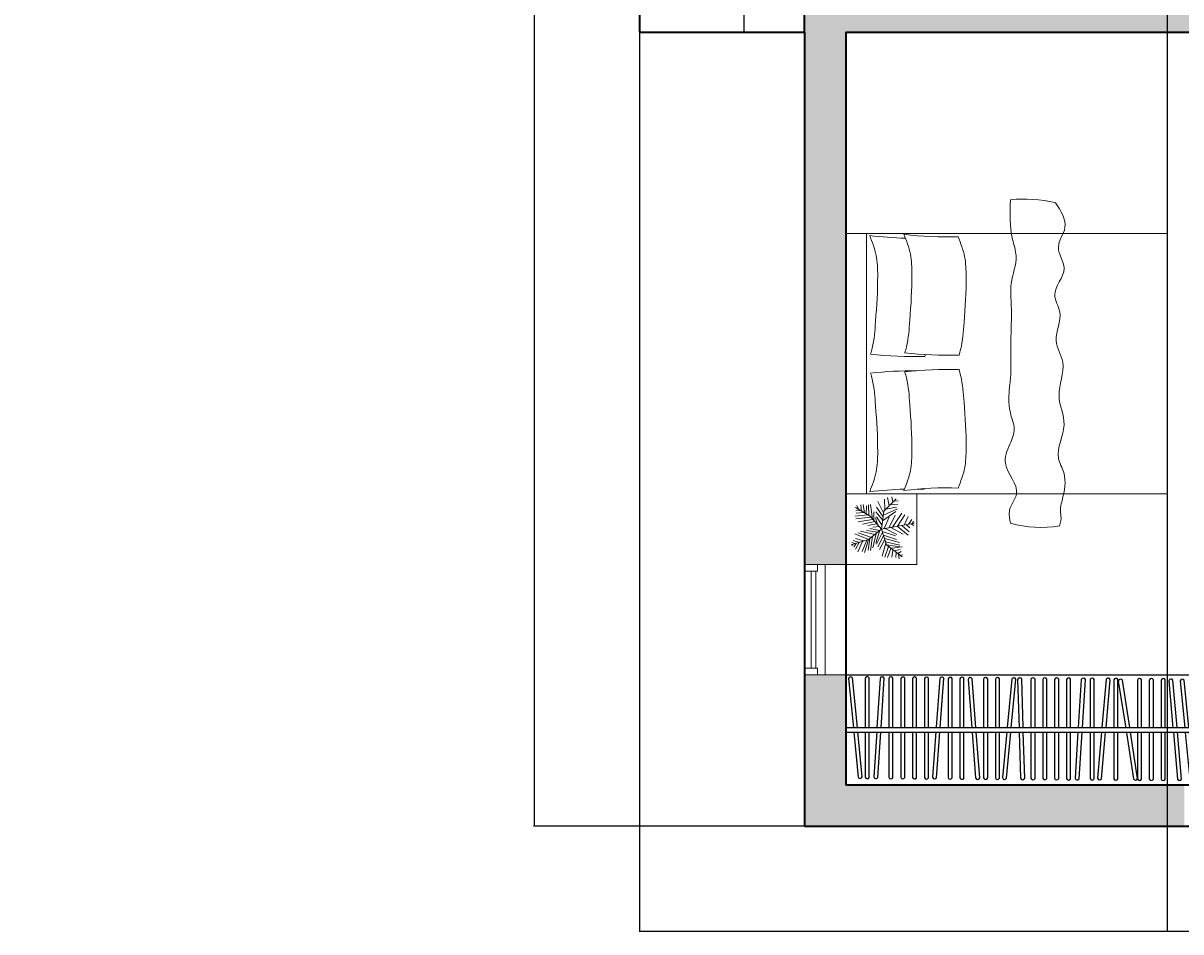
# Model space of a CAD drawing. Units: inches. Extents: x 1789 to 2841, y 3180 to 3702.
# Tile 1 of 14: x 1789 to 2041, y 3180 to 3378. Entities that reach past the tile are written whole.
import ezdxf

# ---------------------------------------------------------------- set-up
doc = ezdxf.new("R2010")
doc.units = ezdxf.units.IN
doc.header["$MEASUREMENT"] = 0
for name, color, linetype, lineweight in [('A-ANNO-DIMS', 2, 'Continuous', 18), ('A-FLOR-CASE', 34, 'Continuous', 25), ('A-WALL', 40, 'Continuous', 35), ('A-WALL-PATT', 252, 'Continuous', 13), ('FURNITURE', 34, 'Continuous', 18), ('WINDOWS', 130, 'Continuous', 18)]:
    doc.layers.add(name, color=color, linetype=linetype, lineweight=lineweight)
doc.styles.get("Standard").update_dxf_attribs({"font": 'arial.ttf'})
doc.dimstyles.get("Standard").update_dxf_attribs({"dimtxt": 0.18, "dimasz": 0.18, "dimexe": 0.18, "dimexo": 0.0625, "dimgap": 0.09, "dimtad": 0, "dimtih": 1, "dimtoh": 1, "dimdec": 0, "dimzin": 0, "dimdsep": 46, "dimlunit": 3, "dimtxsty": 'Standard', "dimcen": 0.09, "dimadec": 0, "dimazin": 0, "dimtfac": 1, "dimtdec": 0, "dimtofl": 0, "dimtmove": 0, "dimatfit": 3, "dimfxl": 1, "dimtolj": 1, "dimtzin": 0, "dimarcsym": 0})

# ---------------------------------------------------------------- blocks, each defined once
blk = doc.blocks.new('CUBOARD')
for p, q in [((2183.73, 3646.16), (2183.73, 3568.16)), ((2184.71, 3646.16), (2184.71, 3568.16))]:
    blk.add_line(p, q)
blk.add_lwpolyline([(2172.23, 3646.16), (2196.23, 3646.16), (2196.23, 3568.16), (2172.23, 3568.16)], close=True)
for points in [[(2183.69, 3644.46), (2173.95, 3643.51)], [(2195.39, 3645.6), (2184.67, 3644.55)], [(2184.76, 3643.66), (2195.54, 3644.71)], [(2195.78, 3645.16), (2195.78, 3645.18)], [(2183.73, 3641.98), (2173.93, 3641.98)], [(2173.97, 3642.61), (2183.78, 3643.57)], [(2195.47, 3641.98), (2184.71, 3641.98)], [(2173.84, 3639.19), (2183.7, 3638.57)], [(2173.86, 3641.08), (2183.73, 3641.08)], [(2183.76, 3639.46), (2173.96, 3640.08)], [(2184.71, 3641.08), (2195.53, 3641.08)], [(2195.45, 3638.71), (2184.74, 3639.4)], [(2195.82, 3641.5), (2195.82, 3641.53)], [(2183.73, 3636.82), (2173.9, 3636.82)], [(2184.68, 3638.5), (2195.46, 3637.81)], [(2195.43, 3636.82), (2184.71, 3636.82)], [(2195.77, 3638.22), (2195.78, 3638.24)], [(2173.83, 3635.92), (2183.73, 3635.92)], [(2183.73, 3634.24), (2173.88, 3634.24)], [(2184.71, 3635.92), (2195.5, 3635.92)], [(2195.42, 3634.24), (2184.71, 3634.24)], [(2195.78, 3636.35), (2195.78, 3636.37)], [(2173.81, 3633.34), (2183.73, 3633.34)], [(2183.73, 3631.66), (2173.86, 3631.66)], [(2184.71, 3633.34), (2195.48, 3633.34)], [(2195.4, 3631.66), (2184.71, 3631.66)], [(2195.77, 3633.77), (2195.77, 3633.79)], [(2173.8, 3630.76), (2183.73, 3630.76)], [(2183.73, 3629.08), (2173.85, 3629.08)], [(2184.71, 3630.76), (2195.47, 3630.76)], [(2195.38, 3629.08), (2184.71, 3629.08)], [(2195.75, 3631.19), (2195.75, 3631.21)], [(2173.78, 3628.19), (2183.73, 3628.19)], [(2183.8, 3626.57), (2173.93, 3627.31)], [(2184.71, 3628.19), (2195.45, 3628.19)], [(2195.4, 3625.7), (2184.78, 3626.5)], [(2195.73, 3628.61), (2195.73, 3628.63)], [(2173.79, 3626.43), (2183.74, 3625.68)], [(2184.71, 3625.61), (2195.4, 3624.81)], [(2195.72, 3625.21), (2195.72, 3625.23)], [(2173.75, 3623.03), (2183.73, 3623.03)], [(2183.73, 3623.92), (2173.81, 3623.92)], [(2195.35, 3623.92), (2184.71, 3623.92)], [(2184.71, 3623.03), (2195.42, 3623.03)], [(2195.7, 3623.45), (2195.7, 3623.48)], [(2173.73, 3620.45), (2183.73, 3620.45)], [(2183.73, 3621.34), (2173.8, 3621.34)], [(2195.22, 3619.57), (2184.65, 3618.76)], [(2195.33, 3621.34), (2184.71, 3621.34)], [(2184.71, 3620.45), (2195.4, 3620.45)], [(2195.6, 3619.13), (2195.6, 3619.15)], [(2195.68, 3620.87), (2195.68, 3620.9)], [(2183.67, 3618.69), (2173.75, 3617.93)], [(2173.75, 3617.03), (2183.74, 3617.8)], [(2184.71, 3617.87), (2195.35, 3618.68)], [(2173.7, 3615.29), (2183.73, 3615.29)], [(2183.73, 3616.19), (2173.77, 3616.19)], [(2195.3, 3616.19), (2184.71, 3616.19)], [(2184.71, 3615.29), (2195.37, 3615.29)], [(2195.65, 3615.71), (2195.65, 3615.74)], [(2173.68, 3612.71), (2183.73, 3612.71)], [(2183.73, 3613.61), (2173.75, 3613.61)], [(2183.78, 3611.12), (2173.82, 3612.07)], [(2195.28, 3613.61), (2184.71, 3613.61)], [(2184.71, 3612.71), (2195.35, 3612.71)], [(2195.63, 3613.14), (2195.63, 3613.16)], [(2173.67, 3611.18), (2183.69, 3610.23)], [(2184.67, 3610.14), (2195.24, 3609.13)], [(2195.26, 3610.03), (2184.75, 3611.03)], [(2195.56, 3609.53), (2195.57, 3609.55)], [(2173.66, 3607.23), (2183.75, 3607.53)], [(2183.72, 3608.42), (2173.71, 3608.13)], [(2195.23, 3608.76), (2184.7, 3608.45)], [(2184.73, 3607.55), (2195.33, 3607.87)], [(2195.6, 3608.3), (2195.6, 3608.32)], [(2173.63, 3604.98), (2183.73, 3604.98)], [(2183.73, 3605.87), (2173.7, 3605.87)], [(2195.23, 3605.87), (2184.71, 3605.87)], [(2184.71, 3604.98), (2195.3, 3604.98)], [(2195.58, 3605.4), (2195.58, 3605.42)], [(2173.61, 3602.4), (2183.73, 3602.4)], [(2183.73, 3603.29), (2173.68, 3603.29)], [(2195.22, 3603.29), (2184.71, 3603.29)], [(2184.71, 3602.4), (2195.28, 3602.4)], [(2195.57, 3602.82), (2195.57, 3602.84)], [(2173.6, 3599.82), (2183.73, 3599.82)], [(2183.73, 3600.71), (2173.67, 3600.71)], [(2195.2, 3600.71), (2184.71, 3600.71)], [(2184.71, 3599.82), (2195.27, 3599.82)], [(2195.55, 3600.24), (2195.55, 3600.27)], [(2173.58, 3597.24), (2183.73, 3597.24)], [(2183.73, 3598.13), (2173.65, 3598.13)], [(2183.77, 3595.62), (2173.68, 3596.25)], [(2195.18, 3598.13), (2184.71, 3598.13)], [(2184.71, 3597.24), (2195.25, 3597.24)], [(2195.53, 3597.66), (2195.53, 3597.69)], [(2173.56, 3595.36), (2183.71, 3594.72)], [(2184.69, 3594.66), (2195.19, 3594)], [(2195.18, 3594.9), (2184.74, 3595.55)], [(2195.5, 3594.4), (2195.5, 3594.43)], [(2173.55, 3592.08), (2183.73, 3592.08)], [(2183.73, 3592.98), (2173.62, 3592.98)], [(2183.73, 3590.49), (2173.72, 3591.37)], [(2195.15, 3592.98), (2184.71, 3592.98)], [(2184.71, 3592.08), (2195.22, 3592.08)], [(2195.5, 3592.5), (2195.5, 3592.53)], [(2173.57, 3590.49), (2183.74, 3589.59)], [(2195.17, 3589.47), (2184.71, 3590.4)], [(2184.71, 3589.5), (2195.16, 3588.58)], [(2195.48, 3588.97), (2195.48, 3589)], [(2173.51, 3586.92), (2183.73, 3586.92)], [(2183.73, 3587.82), (2173.58, 3587.82)], [(2194.84, 3586.83), (2184.58, 3585.23)], [(2195.12, 3587.82), (2184.71, 3587.82)], [(2184.71, 3586.92), (2195.19, 3586.92)], [(2195.26, 3586.41), (2195.25, 3586.44)], [(2195.47, 3587.35), (2195.47, 3587.37)], [(2183.61, 3585.08), (2173.56, 3583.51)], [(2173.63, 3582.62), (2183.75, 3584.19)], [(2184.71, 3584.34), (2195.04, 3585.95)], [(2173.48, 3581.77), (2183.73, 3581.77)], [(2183.73, 3582.66), (2173.55, 3582.66)], [(2195.08, 3582.66), (2184.71, 3582.66)], [(2184.71, 3581.77), (2195.15, 3581.77)], [(2195.43, 3582.19), (2195.43, 3582.21)], [(2173.46, 3579.19), (2183.73, 3579.19)], [(2183.73, 3580.08), (2173.53, 3580.08)], [(2195.07, 3580.08), (2184.71, 3580.08)], [(2184.71, 3579.19), (2195.14, 3579.19)], [(2195.42, 3579.61), (2195.42, 3579.63)], [(2173.45, 3576.61), (2183.73, 3576.61)], [(2183.73, 3577.5), (2173.52, 3577.5)], [(2195.05, 3577.5), (2184.71, 3577.5)], [(2184.71, 3576.61), (2195.12, 3576.61)], [(2195.4, 3577.03), (2195.4, 3577.05)], [(2183.66, 3574.84), (2173.46, 3573.95)], [(2173.47, 3573.05), (2183.74, 3573.94)], [(2194.92, 3575.81), (2184.64, 3574.92)], [(2184.71, 3574.03), (2195.06, 3574.93)], [(2195.31, 3575.37), (2195.31, 3575.4)], [(2183.65, 3572.24), (2173.45, 3571.25)], [(2173.47, 3570.35), (2183.74, 3571.35)], [(2194.88, 3573.34), (2184.63, 3572.34)], [(2184.71, 3571.45), (2195.04, 3572.46)], [(2195.28, 3572.91), (2195.27, 3572.93)], [(2173.4, 3568.87), (2183.73, 3568.87)], [(2183.73, 3569.77), (2173.47, 3569.77)], [(2195, 3569.77), (2184.71, 3569.77)], [(2184.71, 3568.87), (2195.07, 3568.87)], [(2195.35, 3569.29), (2195.35, 3569.32)]]:
    blk.add_lwpolyline(points)
for centre, start, end in [((2195.31, 3645.13), 7.0195, 80.386), ((2195.31, 3645.13), 299.464, 4.1032), ((2174.06, 3641.52), 105.1753, 246.0974), ((2174.12, 3643.06), 110.7367, 251.6587), ((2195.34, 3641.52), 1.4582, 74.8247), ((2174.06, 3639.62), 101.5232, 242.4452), ((2195.34, 3641.52), 293.9026, 358.5418), ((2174.02, 3636.36), 105.1753, 246.0974), ((2195.31, 3636.36), 1.4582, 74.8247), ((2195.3, 3638.26), 357.8061, 71.1726), ((2195.3, 3638.26), 290.2505, 354.8897), ((2174.01, 3633.78), 105.1753, 246.0974), ((2195.29, 3633.78), 1.4582, 74.8247), ((2195.31, 3636.36), 293.9026, 358.5418), ((2173.99, 3631.2), 105.1753, 246.0974), ((2195.27, 3631.2), 1.4582, 74.8247), ((2195.29, 3633.78), 293.9026, 358.5418), ((2173.97, 3628.62), 105.1753, 246.0974), ((2195.26, 3628.62), 1.4582, 74.8247), ((2195.27, 3631.2), 293.9026, 358.5418), ((2174.02, 3626.85), 100.888, 241.81), ((2195.26, 3628.62), 293.9026, 358.5418), ((2195.24, 3625.25), 357.1709, 70.5374), ((2195.24, 3625.25), 289.6153, 354.2545), ((2173.94, 3623.46), 105.1753, 246.0974), ((2195.22, 3623.46), 1.4582, 74.8247), ((2195.22, 3623.46), 293.9026, 358.5418), ((2173.92, 3620.88), 105.1753, 246.0974), ((2195.13, 3619.1), 5.8369, 79.2034), ((2195.21, 3620.88), 1.4582, 74.8247), ((2195.13, 3619.1), 298.2814, 2.9206), ((2195.21, 3620.88), 293.9026, 358.5418), ((2173.9, 3617.48), 109.5541, 250.4761), ((2173.89, 3615.73), 105.1753, 246.0974), ((2195.17, 3615.73), 1.4582, 74.8247), ((2195.17, 3615.73), 293.9026, 358.5418), ((2173.87, 3613.15), 105.1753, 246.0974), ((2173.9, 3611.6), 99.7479, 240.6699), ((2195.16, 3613.15), 1.4582, 74.8247), ((2195.16, 3613.15), 293.9026, 358.5418), ((2195.09, 3609.58), 288.4752, 353.1144), ((2195.09, 3609.58), 356.0307, 69.3973), ((2173.84, 3607.67), 106.858, 247.78), ((2195.12, 3608.3), 3.1408, 76.5073), ((2195.12, 3608.3), 295.5853, 0.2245), ((2173.82, 3605.41), 105.1753, 246.0974), ((2195.11, 3605.41), 1.4582, 74.8247), ((2195.11, 3605.41), 293.9026, 358.5418), ((2173.81, 3602.83), 105.1753, 246.0974), ((2195.09, 3602.83), 1.4582, 74.8247), ((2195.09, 3602.83), 293.9026, 358.5418), ((2173.79, 3600.25), 105.1753, 246.0974), ((2195.08, 3600.25), 1.4582, 74.8247), ((2195.08, 3600.25), 293.9026, 358.5418), ((2173.77, 3597.67), 105.1753, 246.0974), ((2173.78, 3595.78), 101.566, 242.4881), ((2195.06, 3597.67), 1.4582, 74.8247), ((2195.06, 3597.67), 293.9026, 358.5418), ((2195.02, 3594.44), 357.8489, 71.2154), ((2195.02, 3594.44), 290.2933, 354.9325), ((2173.74, 3592.52), 105.1753, 246.0974), ((2173.8, 3590.9), 100.1162, 241.0382), ((2195.03, 3592.52), 1.4582, 74.8247), ((2195.03, 3592.52), 293.9026, 358.5418), ((2195.01, 3589.03), 288.8435, 353.4827), ((2195.01, 3589.03), 356.399, 69.7655), ((2173.71, 3587.36), 105.1753, 246.0974), ((2194.79, 3586.35), 10.3063, 83.6728), ((2194.79, 3586.35), 302.7507, 7.3899), ((2194.99, 3587.36), 1.4582, 74.8247), ((2194.99, 3587.36), 293.9026, 358.5418), ((2173.67, 3582.2), 105.1753, 246.0974), ((2173.75, 3583.08), 114.0234, 254.9455), ((2194.96, 3582.2), 1.4582, 74.8247), ((2194.96, 3582.2), 293.9026, 358.5418), ((2173.66, 3579.62), 105.1753, 246.0974), ((2194.94, 3579.62), 1.4582, 74.8247), ((2194.94, 3579.62), 293.9026, 358.5418), ((2173.64, 3577.04), 105.1753, 246.0974), ((2194.93, 3577.04), 1.4582, 74.8247), ((2194.93, 3577.04), 293.9026, 358.5418), ((2173.63, 3573.5), 110.1314, 251.0534), ((2194.83, 3575.34), 6.4142, 79.7807), ((2194.83, 3575.34), 298.8587, 3.4979), ((2173.62, 3570.8), 110.7648, 251.6868), ((2194.8, 3572.87), 7.0476, 80.4142), ((2194.8, 3572.87), 299.4921, 4.1313), ((2173.59, 3569.31), 105.1753, 246.0974), ((2194.88, 3569.31), 1.4582, 74.8247), ((2194.88, 3569.31), 293.9026, 358.5418)]:
    blk.add_arc(centre, 0.476, start, end)
blk = doc.blocks.new('HY')
for p, q in [((2053.67, 3653.75), (2074.8, 3653.75)), ((2053.67, 3652.75), (2074.8, 3652.75)), ((2052.23, 3650.66), (2076.23, 3650.66))]:
    blk.add_line(p, q)
for points in [[(2076.23, 3646.16), (2052.23, 3646.16), (2052.23, 3655.16), (2076.23, 3655.16)], [(2052.23, 3655.16), (2053.67, 3655.16), (2053.67, 3652.35), (2052.23, 3652.35)], [(2076.23, 3655.16), (2074.8, 3655.16), (2074.8, 3652.35), (2076.23, 3652.35)]]:
    blk.add_lwpolyline(points, close=True)
blk = doc.blocks.new('*U22')
for p, q in [((-5.114, 28.097), (-24.676, 40.636)), ((-7.288, 39.707), (-21.778, 46.673)), ((-8.737, 47.138), (-17.069, 52.711)), ((-10.186, 53.64), (-13.084, 55.962)), ((0, 0), (-10.5, 57)), ((-9.099, 51.782), (-6.563, 55.962)), ((-7.65, 43.423), (-2.578, 49.46)), ((-5.839, 35.992), (4.667, 48.067)), ((-5.114, 27.632), (10.463, 46.673)), ((-31.5, 4.5), (-52.5, 25.5)), ((-48.585, 21.131), (-49.309, 29.026)), ((-43.513, 28.561), (-42.427, 15.558)), ((-38.442, 26.239), (-34.819, 7.663)), ((-35.544, 28.097), (-24.314, 3.947)), ((-14.533, 2.09), (-30.834, 25.31)), ((-3.665, 19.273), (-27.574, 35.527)), ((-24.314, 23.917), (-2.941, 13.7)), ((-2.941, 16.486), (8.652, 37.85)), ((-1.129, 6.734), (9.014, 26.704)), ((3.942, 1.625), (11.187, 24.381)), ((10.101, 3.483), (17.708, 26.239)), ((16.259, 5.805), (23.142, 31.348)), ((22.055, 7.198), (27.489, 32.277)), ((27, 9), (48, 36)), ((27.127, 9.056), (31.112, 35.992)), ((31.836, 30.883), (32.561, 16.486)), ((35.096, 32.741), (37.27, 22.524)), ((38.719, 34.134), (41.979, 28.561)), ((40.53, 25.775), (48.862, 24.846)), ((43.791, 29.954), (51.036, 30.883)), ((44.153, 36.456), (45.239, 32.741)), ((-47.498, 19.737), (-55.83, 18.344)), ((-40.615, 13.7), (-55.105, 10.913)), ((-33.37, 6.269), (-52.207, 5.34)), ((-28.299, 3.483), (-47.86, -5.805)), ((-21.416, 3.018), (-38.079, -8.128)), ((0, 0), (-31.5, 4.5)), ((-15.982, 2.09), (-30.11, -9.521)), ((0, 0), (-22.5, -19.5)), ((-6.563, 1.161), (-21.416, -8.128)), ((-20.691, 13.7), (-1.129, 4.876)), ((0, 0), (27, 9)), ((0, 0), (18, -22.5)), ((6.478, 1.625), (26.04, -8.592)), ((11.187, 3.483), (30.749, -5.805)), ((18.07, 5.805), (35.096, -3.483)), ((24.229, 7.663), (46.688, 1.625)), ((29.662, 12.307), (48.137, 6.269)), ((33.285, 16.486), (48.862, 10.913)), ((36.183, 19.737), (48.137, 17.88)), ((-17.431, -15.094), (-42.789, -18.809)), ((-22.5, -19.5), (-37.5, -45)), ((-15.257, -12.772), (-30.11, -12.772)), ((-20.691, -18.345), (-17.793, -44.352)), ((-6.563, -5.805), (-19.967, -9.985)), ((-17.069, -15.094), (-12.721, -40.172)), ((-13.446, -11.378), (-8.737, -32.741)), ((-9.461, -8.592), (-6.201, -23.453)), ((-4.752, -3.483), (-3.665, -14.629)), ((2.493, -3.019), (-1.491, -20.202)), ((1.769, -2.555), (24.229, -9.521)), ((5.029, -6.27), (2.131, -25.775)), ((9.014, -11.378), (3.58, -35.992)), ((14.085, -16.951), (6.478, -40.172)), ((7.565, -9.056), (32.198, -14.629)), ((12.274, -15.094), (36.907, -18.809)), ((16.259, -19.738), (36.183, -22.989)), ((-28.299, -29.026), (-42.789, -31.348)), ((-24.314, -21.596), (-42.427, -22.06)), ((-30.834, -34.135), (-42.427, -35.528)), ((-34.457, -39.708), (-40.978, -42.494)), ((-26.849, -26.24), (-40.253, -25.775)), ((-32.646, -36.921), (-31.921, -44.352)), ((-29.023, -30.884), (-27.936, -43.887)), ((-25.038, -23.918), (-22.865, -45.281)), ((18.07, -22.524), (8.289, -45.745)), ((20.244, -30.419), (15.897, -44.816)), ((18, -22.5), (27, -52.5)), ((18.433, -22.524), (40.53, -29.026)), ((19.157, -25.311), (38.719, -33.206)), ((22.78, -37.85), (19.519, -48.532)), ((21.331, -32.741), (39.081, -40.636)), ((22.78, -38.314), (34.372, -44.816)), ((24.591, -45.745), (23.142, -50.854)), ((24.591, -43.423), (30.749, -47.603)), ((26.764, -49.925), (28.213, -50.854))]:
    blk.add_line(p, q)
blk = doc.blocks.new('BEDD')
for points in [[(2235.4, 3526.16), (2292.14, 3526.16), (2292.14, 3596.12), (2235.4, 3596.12)], [(2292.14, 3526.16), (2307.57, 3526.16), (2307.57, 3541.59), (2292.14, 3541.59)], [(2235.4, 3526.16), (2292.14, 3526.16), (2292.14, 3530.61), (2235.4, 3530.61)]]:
    blk.add_lwpolyline(points, close=True)
for centre, radius, start, end in [((2259.99, 3564.78), 32.07, 167.4063, 185.0216), ((2273.81, 3568.71), 25.64, 344.9042, 8.8372), ((2163.47, 3548.06), 72.69, 352.674, 2.0029), ((2165.57, 3548.81), 96.38, 354.1175, 1.1854), ((2361.42, 3548.81), 96.38, 178.8146, 185.8825), ((2363.52, 3548.06), 72.69, 177.9971, 187.326), ((2165.85, 3541.35), 96.38, 354.1175, 1.1854), ((2361.69, 3541.35), 96.38, 179.877, 185.8825), ((2363.79, 3540.6), 72.69, 177.9971, 179.1531), ((2163.75, 3540.6), 72.69, 352.674, 358.8312), ((2363.79, 3540.6), 72.69, 181.3344, 187.326)]:
    blk.add_arc(centre, radius, start, end)
for points, knots in [([(2228.7, 3571.77), (2230.5, 3572.97), (2233.69, 3575.11), (2238.44, 3571.24), (2243.48, 3575.3), (2248.08, 3570.3), (2253.24, 3573.93), (2258.37, 3570.76), (2264.15, 3574.63), (2270.52, 3571.37), (2277.36, 3575.01), (2283.2, 3571.25), (2288.29, 3574.45), (2292.59, 3573.51), (2295.73, 3572.7), (2297.56, 3573.17), (2298.4, 3572.89), (2299.15, 3572.65)], [0, 0, 0, 0, 5.813057, 10.291797, 15.071674, 21.264477, 25.062958, 31.395117, 36.284741, 43.6566, 50.0956, 57.47363, 60.824937, 66.871309, 69.965772, 70.260383, 72.512122, 72.512122, 72.512122, 72.512122]), ([(2228.05, 3561.97), (2230.96, 3561.87), (2235.09, 3561.73), (2241.08, 3563.86), (2245.67, 3561.8), (2250.85, 3562.25), (2255.91, 3562.17), (2261.15, 3562), (2265.78, 3562.19), (2270.21, 3561.59), (2274.18, 3561.57), (2278.08, 3563.31), (2281.58, 3561.74), (2286.46, 3559.73), (2291.21, 3564.99), (2295.28, 3561.31), (2297.57, 3561.81), (2298.57, 3562.03)], [0, 0, 0, 0, 8.669632, 12.310458, 18.461416, 22.693385, 27.790985, 33.658819, 38.43562, 41.630677, 47.052462, 50.224855, 53.725722, 58.058029, 65.069701, 68.862462, 71.815525, 71.815525, 71.815525, 71.815525]), ([(2236.12, 3550.6), (2237.54, 3551.15), (2240.34, 3552.23), (2246.72, 3552.46), (2253.43, 3551.99), (2259.2, 3551.57), (2261.51, 3550.92), (2261.93, 3550.8)], [0, 0, 0, 0, 4.544245, 8.926813, 18.957656, 24.819591, 26.148375, 26.148375, 26.148375, 26.148375]), ([(2290.87, 3550.6), (2289.45, 3551.15), (2286.65, 3552.23), (2280.27, 3552.46), (2273.56, 3551.99), (2267.8, 3551.57), (2265.49, 3550.92), (2265.06, 3550.8)], [0, 0, 0, 0, 4.544245, 8.926813, 18.957656, 24.819591, 26.148375, 26.148375, 26.148375, 26.148375]), ([(2235.57, 3538.79), (2236.99, 3539.34), (2239.79, 3540.42), (2246.18, 3540.65), (2252.88, 3540.18), (2258.65, 3539.76), (2260.96, 3539.11), (2261.38, 3538.99)], [0, 0, 0, 0, 4.544245, 8.926813, 18.957656, 24.819591, 26.148375, 26.148375, 26.148375, 26.148375]), ([(2291.42, 3538.79), (2290, 3539.34), (2287.2, 3540.42), (2280.82, 3540.65), (2274.11, 3540.18), (2268.34, 3539.76), (2266.03, 3539.11), (2265.61, 3538.99)], [0, 0, 0, 0, 4.544245, 8.926813, 18.957656, 24.819591, 26.148375, 26.148375, 26.148375, 26.148375]), ([(2235.84, 3531.33), (2237.27, 3531.88), (2240.06, 3532.96), (2246.45, 3533.19), (2253.15, 3532.71), (2258.92, 3532.3), (2261.23, 3531.65), (2261.66, 3531.53)], [0, 0, 0, 0, 4.544245, 8.926813, 18.957656, 24.819591, 26.148375, 26.148375, 26.148375, 26.148375]), ([(2291.69, 3531.33), (2290.27, 3531.88), (2287.47, 3532.96), (2281.09, 3533.19), (2274.39, 3532.71), (2268.62, 3532.3), (2266.31, 3531.65), (2265.88, 3531.53)], [0, 0, 0, 0, 4.544245, 8.926813, 18.957656, 24.819591, 26.148375, 26.148375, 26.148375, 26.148375])]:
    blk.add_open_spline(points, degree=3, knots=knots)
for points in [[(2261.81, 3543.46), (2261.94, 3543.42), (2262.07, 3543.38), (2262.21, 3543.34)], [(2291.15, 3543.14), (2291.09, 3543.16), (2291.04, 3543.18), (2290.99, 3543.2)]]:
    blk.add_open_spline(points, degree=3)
at = {"xscale": 0.1258179792922857, "yscale": 0.1258179792922857, "zscale": 0.1258179792922857}
blk.add_blockref('*U22', (2299.85, 3533.87), dxfattribs=at)
blk = doc.blocks.new('*D79')
at = {"layer": 'A-ANNO-DIMS', "color": 0, "lineweight": -2, "transparency": 16777216}
for p, q in [((1923.23, 3376.1), (1923.23, 3180.13)), ((2325.23, 3203.1), (2325.23, 3180.13)), ((1923.41, 3180.31), (2123.94, 3180.31)), ((2325.05, 3180.31), (2124.52, 3180.31))]:
    blk.add_line(p, q, dxfattribs=at)
at = {"layer": 'A-ANNO-DIMS', "color": 0, "transparency": 16777216}
for points in [[(1923.41, 3180.34), (1923.41, 3180.28), (1923.23, 3180.31)], [(2325.05, 3180.34), (2325.05, 3180.28), (2325.23, 3180.31)]]:
    blk.add_solid(points, dxfattribs=at)
at = {"layer": 'Defpoints', "color": 0, "transparency": 16777216}
for p in [(1923.23, 3376.16), (2325.23, 3203.16), (2325.23, 3180.31)]:
    blk.add_point(p, dxfattribs=at)
at = {"layer": 'A-ANNO-DIMS', "color": 0, "transparency": 16777216, "insert": (2124.23, 3180.31), "char_height": 0.18, "attachment_point": 5}
blk.add_mtext('\\A1;402', dxfattribs=at)
blk = doc.blocks.new('*D80')
at = {"layer": 'A-ANNO-DIMS', "color": 0, "lineweight": -2, "transparency": 16777216}
for p, q in [((1959.17, 3655.16), (1900.2, 3655.16)), ((1900.38, 3654.98), (1900.38, 3429.34)), ((1900.38, 3203.34), (1900.38, 3428.98)), ((1959.17, 3203.16), (1900.2, 3203.16))]:
    blk.add_line(p, q, dxfattribs=at)
at = {"layer": 'A-ANNO-DIMS', "color": 0, "transparency": 16777216}
for points in [[(1900.35, 3654.98), (1900.41, 3654.98), (1900.38, 3655.16)], [(1900.35, 3203.34), (1900.41, 3203.34), (1900.38, 3203.16)]]:
    blk.add_solid(points, dxfattribs=at)
at = {"layer": 'Defpoints', "color": 0, "transparency": 16777216}
for p in [(1959.23, 3655.16), (1900.38, 3203.16), (1959.23, 3203.16)]:
    blk.add_point(p, dxfattribs=at)
at = {"layer": 'A-ANNO-DIMS', "color": 0, "transparency": 16777216, "insert": (1900.38, 3429.16), "char_height": 0.18, "attachment_point": 5}
blk.add_mtext('\\A1;452', dxfattribs=at)
blk = doc.blocks.new('*D90')
at = {"layer": 'A-ANNO-DIMS', "color": 0, "lineweight": -2, "transparency": 16777216}
for p, q in [((2038.23, 3517.1), (2038.23, 3180.13)), ((2074.23, 3517.1), (2074.23, 3180.13)), ((2038.41, 3180.31), (2056.01, 3180.31)), ((2074.05, 3180.31), (2056.45, 3180.31))]:
    blk.add_line(p, q, dxfattribs=at)
at = {"layer": 'A-ANNO-DIMS', "color": 0, "transparency": 16777216}
for points in [[(2038.41, 3180.34), (2038.41, 3180.28), (2038.23, 3180.31)], [(2074.05, 3180.34), (2074.05, 3180.28), (2074.23, 3180.31)]]:
    blk.add_solid(points, dxfattribs=at)
at = {"layer": 'Defpoints', "color": 0, "transparency": 16777216}
for p in [(2038.23, 3517.16), (2074.23, 3517.16), (2074.23, 3180.31)]:
    blk.add_point(p, dxfattribs=at)
at = {"layer": 'A-ANNO-DIMS', "color": 0, "transparency": 16777216, "insert": (2056.23, 3180.31), "char_height": 0.18, "attachment_point": 5}
blk.add_mtext('\\A1;36', dxfattribs=at)
blk = doc.blocks.new('*D94')
at = {"layer": 'A-ANNO-DIMS', "color": 0, "lineweight": -2, "transparency": 16777216}
for p, q in [((1923.3, 3483.69), (1946.26, 3483.69)), ((1946.08, 3483.51), (1946.08, 3430.11)), ((1946.08, 3376.34), (1946.08, 3429.74)), ((1923.3, 3376.16), (1946.26, 3376.16))]:
    blk.add_line(p, q, dxfattribs=at)
at = {"layer": 'A-ANNO-DIMS', "color": 0, "transparency": 16777216}
for points in [[(1946.05, 3483.51), (1946.11, 3483.51), (1946.08, 3483.69)], [(1946.05, 3376.34), (1946.11, 3376.34), (1946.08, 3376.16)]]:
    blk.add_solid(points, dxfattribs=at)
at = {"layer": 'Defpoints', "color": 0, "transparency": 16777216}
for p in [(1923.23, 3483.69), (1923.23, 3376.16), (1946.08, 3376.16)]:
    blk.add_point(p, dxfattribs=at)
at = {"layer": 'A-ANNO-DIMS', "color": 0, "transparency": 16777216, "insert": (1946.08, 3429.92), "char_height": 0.18, "attachment_point": 5}
blk.add_mtext('\\A1;107.53', dxfattribs=at)
blk = doc.blocks.new('*D116')
at = {"layer": 'A-ANNO-DIMS', "color": 0, "lineweight": -2, "transparency": 16777216}
for p, q in [((1789.65, 3701.85), (1789.83, 3701.85)), ((1789.83, 3701.85), (1945.65, 3528.3)), ((2205.56, 3238.68), (2205.74, 3238.68)), ((2205.65, 3238.59), (2205.65, 3238.77))]:
    blk.add_line(p, q, dxfattribs=at)
at = {"layer": 'A-ANNO-DIMS', "color": 0, "transparency": 16777216}
blk.add_solid([(1945.67, 3528.32), (1945.62, 3528.28), (1945.77, 3528.16)], dxfattribs=at)
at = {"layer": 'Defpoints', "color": 0, "transparency": 16777216}
for p in [(1945.77, 3528.16), (2205.65, 3238.68)]:
    blk.add_point(p, dxfattribs=at)
at = {"layer": 'A-ANNO-DIMS', "color": 0, "transparency": 16777216, "insert": (1789.28, 3701.85), "char_height": 0.18, "attachment_point": 5}
blk.add_mtext('\\A1;R389', dxfattribs=at)

msp = doc.modelspace()

# ---------------------------------------------------------------- hatches: boundary and pattern name
at = {"layer": 'A-WALL-PATT'}
h = msp.add_hatch(color=256, dxfattribs=at)
h.dxf.hatch_style = 1
h.paths.add_polyline_path([(1968.2333, 3376.1608), (2072.0492, 3376.1608, -0.02086055), (2071.924, 3379.1608), (2071.924, 3385.1608), (2001.2333, 3385.1608), (2001.2333, 3413.9882), (1992.2333, 3413.9882), (1992.2333, 3385.1608), (1968.3016, 3385.1608), (1959.2333, 3385.1608), (1959.2333, 3376.1608), (1959.2333, 3260.1608), (1968.2333, 3260.1608), (1968.2333, 3275.5886), (1968.2333, 3332.3251)])
h = msp.add_hatch(color=256, dxfattribs=at)
h.dxf.hatch_style = 1
h.paths.add_polyline_path([(2154.3707, 3212.1608), (2121.2333, 3212.1608), (2121.2333, 3216.7108), (2121.2333, 3239.3636, -0.02504709), (2118.2333, 3239.2132), (2112.2333, 3239.2132), (2112.2333, 3212.1608), (2101.9504, 3212.1608), (2101.9504, 3203.1608), (2154.3707, 3203.1608)])
h.paths.add_polyline_path([(2041.9504, 3212.1608), (1968.2333, 3212.1608), (1968.2333, 3236.1608), (1959.2333, 3236.1608), (1959.2333, 3203.1608), (2041.9504, 3203.1608)])

# ---------------------------------------------------------------- linework, layer by layer
at = {"layer": 'A-WALL'}
for p, q in [((1923.2333, 3483.6885), (1923.2333, 3376.1608)), ((1959.2333, 3376.1608), (1959.2333, 3385.1608)), ((1923.2333, 3376.1608), (1959.2333, 3376.1608)), ((1959.2333, 3376.1608), (1959.2333, 3203.1608)), ((1968.2333, 3376.1608), (1968.2333, 3212.1608)), ((1968.2333, 3376.1608), (2072.0492, 3376.1608)), ((1968.2333, 3212.1608), (2112.2333, 3212.1608)), ((1959.2333, 3203.1608), (2325.2333, 3203.1608))]:
    msp.add_line(p, q, dxfattribs=at)

# ---------------------------------------------------------------- block references
at = {"layer": 'A-FLOR-CASE', "rotation": 90}
msp.add_blockref('CUBOARD', (5614.3941, 1039.9274), dxfattribs=at)
at = {"layer": 'FURNITURE', "rotation": 270}
msp.add_blockref('BEDD', (-1557.9274, 5567.7261), dxfattribs=at)
at = {"layer": 'WINDOWS', "rotation": 89.99999999999999}
msp.add_blockref('HY', (5614.3941, 1183.9274), dxfattribs=at)

# ---------------------------------------------------------------- dimensions: what is measured, and where the dimension line sits
at = {"layer": 'A-ANNO-DIMS'}
dim = msp.add_radius_dim(center=(2205.6545, 3238.6823), mpoint=(1945.766, 3528.162), dimstyle='Standard', override={"dimdec": 0, "dimlfac": 1, "dimrnd": 0, "dimzin": 0, "dimdsep": 46, "dimlunit": 2}, dxfattribs=at)
dim.commit()
dim.dimension.update_dxf_attribs({"geometry": '*D116', "text_midpoint": (1789.2778, 3701.8498), "dimtype": 164})
for base, p1, p2, angle, override, picture, middle in [((1900.3833, 3203.1608), (1959.2333, 3655.1608), (1959.2333, 3203.1608), 90, {"dimdec": 0, "dimlfac": 1, "dimrnd": 0, "dimzin": 0, "dimdsep": 46, "dimlunit": 2}, '*D80', (1900.3833, 3429.1608)), ((1946.0833, 3376.1608), (1923.2333, 3483.6885), (1923.2333, 3376.1608), 270, {"dimdec": 2, "dimlfac": 1, "dimrnd": 0, "dimzin": 0, "dimdsep": 46, "dimlunit": 2}, '*D94', (1946.0833, 3429.9246))]:
    dim = msp.add_linear_dim(base=base, p1=p1, p2=p2, angle=angle, dimstyle='Standard', override=override, dxfattribs=at)
    dim.commit()
    dim.dimension.update_dxf_attribs({"geometry": picture, "text_midpoint": middle})
for base, p1, p2, picture, middle in [((2074.2333, 3180.3108), (2038.2333, 3517.1608), (2074.2333, 3517.1608), '*D90', (2056.2333, 3180.3108)), ((2325.2333, 3180.3108), (1923.2333, 3376.1608), (2325.2333, 3203.1608), '*D79', (2124.2333, 3180.3108))]:
    dim = msp.add_linear_dim(base=base, p1=p1, p2=p2, dimstyle='Standard', override={"dimdec": 0, "dimlfac": 1, "dimrnd": 0, "dimzin": 0, "dimdsep": 46, "dimlunit": 2}, dxfattribs=at)
    dim.commit()
    dim.dimension.update_dxf_attribs({"geometry": picture, "text_midpoint": middle})

doc.saveas('drawing.dxf')
